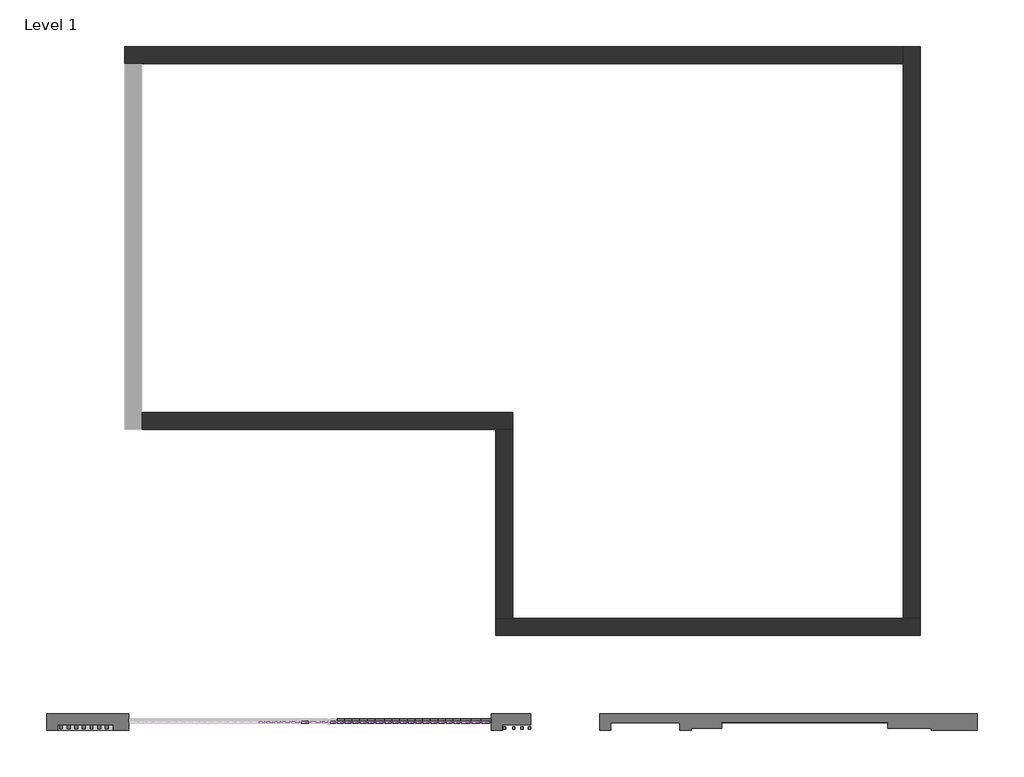
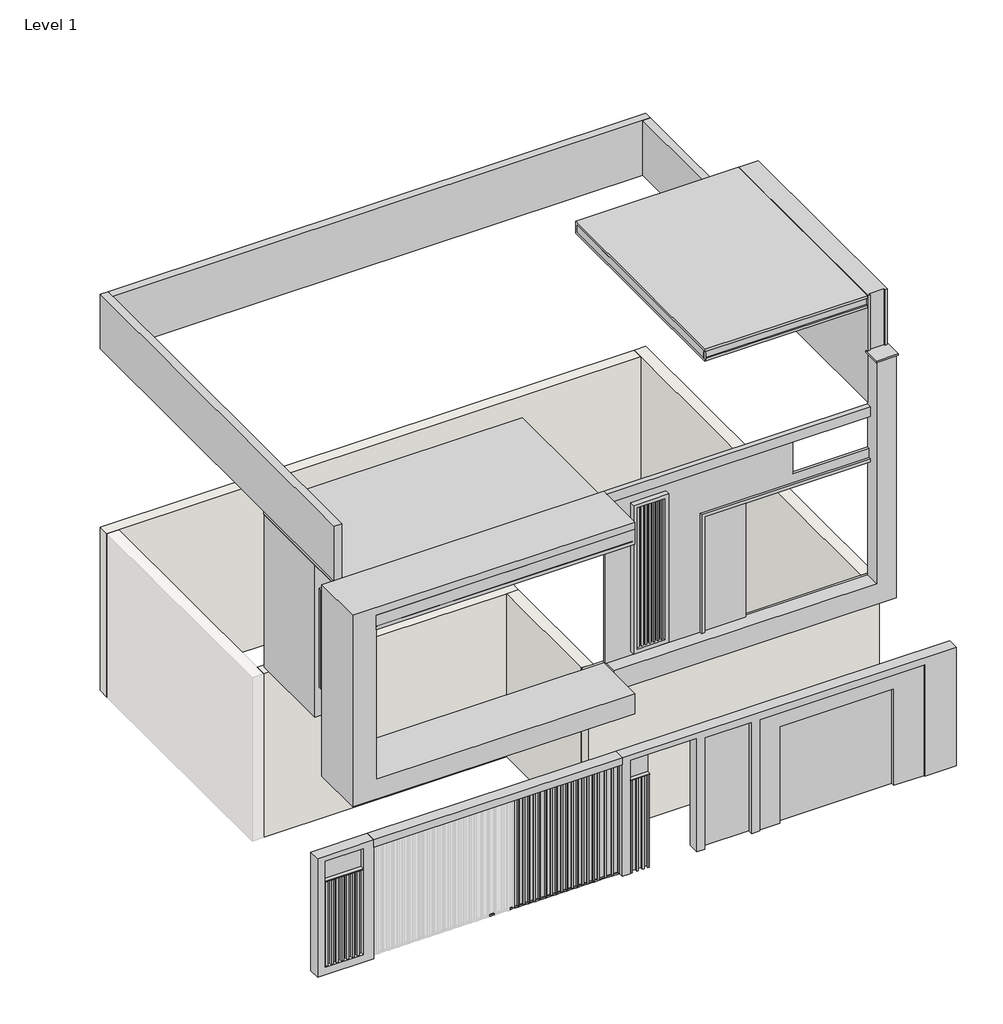
# One storey, part 2 of 2: 68 members, 19 plates, 5 walls, 1 proxy.
"""IFC4 building model written with IfcOpenShell, lengths in millimetres."""

from ifc_helpers import new_model, si_unit, frame, origin, place, context, project, spatial, polyline, outline, extrude, faceted_brep, transform, mapped, element, save
from components import generic_models_1_generic_models_1_ed2606db, member_dc9417da, member_f9b59f6e, member_b36ee676, member_838ad8ec, member_d2c643f7, member_fc53d4cb, member_4ec4fa50, member_7046656e, system_panel_glazed_eef689be, system_panel_glazed_28c5fff6, system_panel_glazed_b538bb1a

model = new_model("IFC4")

# Units and contexts
model_context = context("Model", 3, world=origin())
ifc_project = project(units=[si_unit("LENGTHUNIT", "METRE", prefix="MILLI")], contexts=[model_context])

# Site, building, storey
site = spatial("IfcSite", under=ifc_project)
building = spatial("IfcBuilding", under=site)
storey = spatial("IfcBuildingStorey", under=building, Name="Level 1", Elevation=-304.8)

# Proxy
placement = place(None, origin())
generic_models_1_generic_models_1_shape = generic_models_1_generic_models_1_ed2606db(model_context)
element("IfcBuildingElementProxy", 1, Name="Generic Models 1 : Generic Models 1", ObjectType="Generic Models 1 : Generic Models 1", at=placement, inside=storey, context=model_context, shape_type="MappedRepresentation", body=[
    mapped(generic_models_1_generic_models_1_shape, transform((0.0, 0.0, 0.0), x_axis=(1.0, 0.0, 0.0), y_axis=(0.0, 1.0, 0.0), z_axis=(0.0, 0.0, 1.0))),
])

# Members
member_shape = member_dc9417da(model_context)
element("IfcMember", 2, ObjectType="Rectangular Mullion : 1\" Square", at=placement, inside=storey, context=model_context, shape_type="MappedRepresentation", body=[
    mapped(member_shape, transform((-5007.1379854, -6958.7165974, 1982.7875), x_axis=(0.0, 0.0, 1.0), y_axis=(0.0, -1.0, 0.0), z_axis=(1.0, 0.0, 0.0))),
])
member_2_shape = member_f9b59f6e(model_context)
element("IfcMember", 3, ObjectType="Rectangular Mullion : 1\" Square", at=placement, inside=storey, context=model_context, shape_type="MappedRepresentation", body=[
    mapped(member_2_shape, transform((-6937.5379854, -6958.7165974, -304.8), x_axis=(1.0, 0.0, 0.0), y_axis=(0.0, -1.0, 0.0), z_axis=(0.0, 0.0, -1.0))),
])
element("IfcMember", 4, ObjectType="Rectangular Mullion : 1\" Square", at=placement, inside=storey, context=model_context, shape_type="MappedRepresentation", body=[
    mapped(member_2_shape, transform((-6835.9379854, -6958.7165974, -304.8), x_axis=(1.0, 0.0, 0.0), y_axis=(0.0, -1.0, 0.0), z_axis=(0.0, 0.0, -1.0))),
])
element("IfcMember", 5, ObjectType="Rectangular Mullion : 1\" Square", at=placement, inside=storey, context=model_context, shape_type="MappedRepresentation", body=[
    mapped(member_2_shape, transform((-6734.3379854, -6958.7165974, -304.8), x_axis=(1.0, 0.0, 0.0), y_axis=(0.0, -1.0, 0.0), z_axis=(0.0, 0.0, -1.0))),
])
element("IfcMember", 6, ObjectType="Rectangular Mullion : 1\" Square", at=placement, inside=storey, context=model_context, shape_type="MappedRepresentation", body=[
    mapped(member_2_shape, transform((-6632.7379854, -6958.7165974, -304.8), x_axis=(1.0, 0.0, 0.0), y_axis=(0.0, -1.0, 0.0), z_axis=(0.0, 0.0, -1.0))),
])
element("IfcMember", 7, ObjectType="Rectangular Mullion : 1\" Square", at=placement, inside=storey, context=model_context, shape_type="MappedRepresentation", body=[
    mapped(member_2_shape, transform((-6531.1379854, -6958.7165974, -304.8), x_axis=(1.0, 0.0, 0.0), y_axis=(0.0, -1.0, 0.0), z_axis=(0.0, 0.0, -1.0))),
])
element("IfcMember", 8, ObjectType="Rectangular Mullion : 1\" Square", at=placement, inside=storey, context=model_context, shape_type="MappedRepresentation", body=[
    mapped(member_2_shape, transform((-6404.1379854, -6958.7165974, -304.8), x_axis=(1.0, 0.0, 0.0), y_axis=(0.0, -1.0, 0.0), z_axis=(0.0, 0.0, -1.0))),
])
element("IfcMember", 9, ObjectType="Rectangular Mullion : 1\" Square", at=placement, inside=storey, context=model_context, shape_type="MappedRepresentation", body=[
    mapped(member_2_shape, transform((-6302.5379854, -6958.7165974, -304.8), x_axis=(1.0, 0.0, 0.0), y_axis=(0.0, -1.0, 0.0), z_axis=(0.0, 0.0, -1.0))),
])
element("IfcMember", 10, ObjectType="Rectangular Mullion : 1\" Square", at=placement, inside=storey, context=model_context, shape_type="MappedRepresentation", body=[
    mapped(member_2_shape, transform((-6200.9379854, -6958.7165974, -304.8), x_axis=(1.0, 0.0, 0.0), y_axis=(0.0, -1.0, 0.0), z_axis=(0.0, 0.0, -1.0))),
])
element("IfcMember", 11, ObjectType="Rectangular Mullion : 1\" Square", at=placement, inside=storey, context=model_context, shape_type="MappedRepresentation", body=[
    mapped(member_2_shape, transform((-6099.3379854, -6958.7165974, -304.8), x_axis=(1.0, 0.0, 0.0), y_axis=(0.0, -1.0, 0.0), z_axis=(0.0, 0.0, -1.0))),
])
element("IfcMember", 12, ObjectType="Rectangular Mullion : 1\" Square", at=placement, inside=storey, context=model_context, shape_type="MappedRepresentation", body=[
    mapped(member_2_shape, transform((-5997.7379854, -6958.7165974, -304.8), x_axis=(1.0, 0.0, 0.0), y_axis=(0.0, -1.0, 0.0), z_axis=(0.0, 0.0, -1.0))),
])
element("IfcMember", 13, ObjectType="Rectangular Mullion : 1\" Square", at=placement, inside=storey, context=model_context, shape_type="MappedRepresentation", body=[
    mapped(member_2_shape, transform((-5896.1379854, -6958.7165974, -304.8), x_axis=(1.0, 0.0, 0.0), y_axis=(0.0, -1.0, 0.0), z_axis=(0.0, 0.0, -1.0))),
])
element("IfcMember", 14, ObjectType="Rectangular Mullion : 1\" Square", at=placement, inside=storey, context=model_context, shape_type="MappedRepresentation", body=[
    mapped(member_2_shape, transform((-5794.5379854, -6958.7165974, -304.8), x_axis=(1.0, 0.0, 0.0), y_axis=(0.0, -1.0, 0.0), z_axis=(0.0, 0.0, -1.0))),
])
element("IfcMember", 15, ObjectType="Rectangular Mullion : 1\" Square", at=placement, inside=storey, context=model_context, shape_type="MappedRepresentation", body=[
    mapped(member_2_shape, transform((-5692.9379854, -6958.7165974, -304.8), x_axis=(1.0, 0.0, 0.0), y_axis=(0.0, -1.0, 0.0), z_axis=(0.0, 0.0, -1.0))),
])
element("IfcMember", 16, ObjectType="Rectangular Mullion : 1\" Square", at=placement, inside=storey, context=model_context, shape_type="MappedRepresentation", body=[
    mapped(member_2_shape, transform((-5591.3379854, -6958.7165974, -304.8), x_axis=(1.0, 0.0, 0.0), y_axis=(0.0, -1.0, 0.0), z_axis=(0.0, 0.0, -1.0))),
])
element("IfcMember", 17, ObjectType="Rectangular Mullion : 1\" Square", at=placement, inside=storey, context=model_context, shape_type="MappedRepresentation", body=[
    mapped(member_2_shape, transform((-5489.7379854, -6958.7165974, -304.8), x_axis=(1.0, 0.0, 0.0), y_axis=(0.0, -1.0, 0.0), z_axis=(0.0, 0.0, -1.0))),
])
element("IfcMember", 18, ObjectType="Rectangular Mullion : 1\" Square", at=placement, inside=storey, context=model_context, shape_type="MappedRepresentation", body=[
    mapped(member_2_shape, transform((-5388.1379854, -6958.7165974, -304.8), x_axis=(1.0, 0.0, 0.0), y_axis=(0.0, -1.0, 0.0), z_axis=(0.0, 0.0, -1.0))),
])
element("IfcMember", 19, ObjectType="Rectangular Mullion : 1\" Square", at=placement, inside=storey, context=model_context, shape_type="MappedRepresentation", body=[
    mapped(member_2_shape, transform((-5252.6713187, -6958.7165974, -304.8), x_axis=(1.0, 0.0, 0.0), y_axis=(0.0, -1.0, 0.0), z_axis=(0.0, 0.0, -1.0))),
])
element("IfcMember", 20, ObjectType="Rectangular Mullion : 1\" Square", at=placement, inside=storey, context=model_context, shape_type="MappedRepresentation", body=[
    mapped(member_2_shape, transform((-5117.204652, -6958.7165974, -304.8), x_axis=(1.0, 0.0, 0.0), y_axis=(0.0, -1.0, 0.0), z_axis=(0.0, 0.0, -1.0))),
])
member_3_shape = member_b36ee676(model_context)
element("IfcMember", 21, ObjectType="Rectangular Mullion : 1\" Square", at=placement, inside=storey, context=model_context, shape_type="MappedRepresentation", body=[
    mapped(member_3_shape, transform((-7121.6879854, -6958.7165974, -304.8), x_axis=(0.0, 0.0, -1.0), y_axis=(0.0, -1.0, 0.0), z_axis=(-1.0, 0.0, 0.0))),
])
member_4_shape = member_838ad8ec(model_context)
element("IfcMember", 22, ObjectType="Rectangular Mullion : 1\" Square", at=placement, inside=storey, context=model_context, shape_type="MappedRepresentation", body=[
    mapped(member_4_shape, transform((-7026.4379854, -6958.7165974, -304.8), x_axis=(0.0, 0.0, -1.0), y_axis=(0.0, -1.0, 0.0), z_axis=(-1.0, 0.0, 0.0))),
])
element("IfcMember", 23, ObjectType="Rectangular Mullion : 1\" Square", at=placement, inside=storey, context=model_context, shape_type="MappedRepresentation", body=[
    mapped(member_4_shape, transform((-6924.8379854, -6958.7165974, -304.8), x_axis=(0.0, 0.0, -1.0), y_axis=(0.0, -1.0, 0.0), z_axis=(-1.0, 0.0, 0.0))),
])
element("IfcMember", 24, ObjectType="Rectangular Mullion : 1\" Square", at=placement, inside=storey, context=model_context, shape_type="MappedRepresentation", body=[
    mapped(member_4_shape, transform((-6823.2379854, -6958.7165974, -304.8), x_axis=(0.0, 0.0, -1.0), y_axis=(0.0, -1.0, 0.0), z_axis=(-1.0, 0.0, 0.0))),
])
element("IfcMember", 25, ObjectType="Rectangular Mullion : 1\" Square", at=placement, inside=storey, context=model_context, shape_type="MappedRepresentation", body=[
    mapped(member_4_shape, transform((-6721.6379854, -6958.7165974, -304.8), x_axis=(0.0, 0.0, -1.0), y_axis=(0.0, -1.0, 0.0), z_axis=(-1.0, 0.0, 0.0))),
])
element("IfcMember", 26, ObjectType="Rectangular Mullion : 1\" Square", at=placement, inside=storey, context=model_context, shape_type="MappedRepresentation", body=[
    mapped(member_4_shape, transform((-6620.0379854, -6958.7165974, -304.8), x_axis=(0.0, 0.0, -1.0), y_axis=(0.0, -1.0, 0.0), z_axis=(-1.0, 0.0, 0.0))),
])
element("IfcMember", 27, ObjectType="Rectangular Mullion : 1\" Square", at=placement, inside=storey, context=model_context, shape_type="MappedRepresentation", body=[
    mapped(member_4_shape, transform((-6391.4379854, -6958.7165974, -304.8), x_axis=(0.0, 0.0, -1.0), y_axis=(0.0, -1.0, 0.0), z_axis=(-1.0, 0.0, 0.0))),
])
element("IfcMember", 28, ObjectType="Rectangular Mullion : 1\" Square", at=placement, inside=storey, context=model_context, shape_type="MappedRepresentation", body=[
    mapped(member_4_shape, transform((-6289.8379854, -6958.7165974, -304.8), x_axis=(0.0, 0.0, -1.0), y_axis=(0.0, -1.0, 0.0), z_axis=(-1.0, 0.0, 0.0))),
])
element("IfcMember", 29, ObjectType="Rectangular Mullion : 1\" Square", at=placement, inside=storey, context=model_context, shape_type="MappedRepresentation", body=[
    mapped(member_4_shape, transform((-6188.2379854, -6958.7165974, -304.8), x_axis=(0.0, 0.0, -1.0), y_axis=(0.0, -1.0, 0.0), z_axis=(-1.0, 0.0, 0.0))),
])
element("IfcMember", 30, ObjectType="Rectangular Mullion : 1\" Square", at=placement, inside=storey, context=model_context, shape_type="MappedRepresentation", body=[
    mapped(member_4_shape, transform((-6086.6379854, -6958.7165974, -304.8), x_axis=(0.0, 0.0, -1.0), y_axis=(0.0, -1.0, 0.0), z_axis=(-1.0, 0.0, 0.0))),
])
element("IfcMember", 31, ObjectType="Rectangular Mullion : 1\" Square", at=placement, inside=storey, context=model_context, shape_type="MappedRepresentation", body=[
    mapped(member_4_shape, transform((-5985.0379854, -6958.7165974, -304.8), x_axis=(0.0, 0.0, -1.0), y_axis=(0.0, -1.0, 0.0), z_axis=(-1.0, 0.0, 0.0))),
])
element("IfcMember", 32, ObjectType="Rectangular Mullion : 1\" Square", at=placement, inside=storey, context=model_context, shape_type="MappedRepresentation", body=[
    mapped(member_4_shape, transform((-5883.4379854, -6958.7165974, -304.8), x_axis=(0.0, 0.0, -1.0), y_axis=(0.0, -1.0, 0.0), z_axis=(-1.0, 0.0, 0.0))),
])
element("IfcMember", 33, ObjectType="Rectangular Mullion : 1\" Square", at=placement, inside=storey, context=model_context, shape_type="MappedRepresentation", body=[
    mapped(member_4_shape, transform((-5781.8379854, -6958.7165974, -304.8), x_axis=(0.0, 0.0, -1.0), y_axis=(0.0, -1.0, 0.0), z_axis=(-1.0, 0.0, 0.0))),
])
element("IfcMember", 34, ObjectType="Rectangular Mullion : 1\" Square", at=placement, inside=storey, context=model_context, shape_type="MappedRepresentation", body=[
    mapped(member_4_shape, transform((-5680.2379854, -6958.7165974, -304.8), x_axis=(0.0, 0.0, -1.0), y_axis=(0.0, -1.0, 0.0), z_axis=(-1.0, 0.0, 0.0))),
])
element("IfcMember", 35, ObjectType="Rectangular Mullion : 1\" Square", at=placement, inside=storey, context=model_context, shape_type="MappedRepresentation", body=[
    mapped(member_4_shape, transform((-5578.6379854, -6958.7165974, -304.8), x_axis=(0.0, 0.0, -1.0), y_axis=(0.0, -1.0, 0.0), z_axis=(-1.0, 0.0, 0.0))),
])
element("IfcMember", 36, ObjectType="Rectangular Mullion : 1\" Square", at=placement, inside=storey, context=model_context, shape_type="MappedRepresentation", body=[
    mapped(member_4_shape, transform((-5477.0379854, -6958.7165974, -304.8), x_axis=(0.0, 0.0, -1.0), y_axis=(0.0, -1.0, 0.0), z_axis=(-1.0, 0.0, 0.0))),
])
member_5_shape = member_d2c643f7(model_context)
element("IfcMember", 37, ObjectType="Rectangular Mullion : 1\" Square", at=placement, inside=storey, context=model_context, shape_type="MappedRepresentation", body=[
    mapped(member_5_shape, transform((-7509.0379854, -6958.7165974, -304.8), x_axis=(0.0, 0.0, -1.0), y_axis=(0.0, -1.0, 0.0), z_axis=(-1.0, 0.0, 0.0))),
])
element("IfcMember", 38, ObjectType="Rectangular Mullion : 1\" Square", at=placement, inside=storey, context=model_context, shape_type="MappedRepresentation", body=[
    mapped(member_5_shape, transform((-6518.4379854, -6958.7165974, -304.8), x_axis=(0.0, 0.0, -1.0), y_axis=(0.0, -1.0, 0.0), z_axis=(-1.0, 0.0, 0.0))),
])
member_6_shape = member_fc53d4cb(model_context)
element("IfcMember", 39, ObjectType="Rectangular Mullion : 1\" Square", at=placement, inside=storey, context=model_context, shape_type="MappedRepresentation", body=[
    mapped(member_6_shape, transform((-5375.4379854, -6958.7165974, -304.8), x_axis=(0.0, 0.0, -1.0), y_axis=(0.0, -1.0, 0.0), z_axis=(-1.0, 0.0, 0.0))),
])
element("IfcMember", 40, ObjectType="Rectangular Mullion : 1\" Square", at=placement, inside=storey, context=model_context, shape_type="MappedRepresentation", body=[
    mapped(member_6_shape, transform((-5239.9713187, -6958.7165974, -304.8), x_axis=(0.0, 0.0, -1.0), y_axis=(0.0, -1.0, 0.0), z_axis=(-1.0, 0.0, 0.0))),
])
element("IfcMember", 41, ObjectType="Rectangular Mullion : 1\" Square", at=placement, inside=storey, context=model_context, shape_type="MappedRepresentation", body=[
    mapped(member_shape, transform((-5104.504652, -6958.7165974, -304.8), x_axis=(0.0, 0.0, -1.0), y_axis=(0.0, -1.0, 0.0), z_axis=(-1.0, 0.0, 0.0))),
])
element("IfcMember", 42, ObjectType="Rectangular Mullion : 1\" Square", at=placement, inside=storey, context=model_context, shape_type="MappedRepresentation", body=[
    mapped(member_5_shape, transform((-7407.4379854, -6958.7165974, 1982.7875), x_axis=(0.0, 0.0, 1.0), y_axis=(0.0, -1.0, 0.0), z_axis=(1.0, 0.0, 0.0))),
])
element("IfcMember", 43, ObjectType="Rectangular Mullion : 1\" Square", at=placement, inside=storey, context=model_context, shape_type="MappedRepresentation", body=[
    mapped(member_5_shape, transform((-7661.4379854, -6958.7165974, 1982.7875), x_axis=(0.0, 0.0, 1.0), y_axis=(0.0, -1.0, 0.0), z_axis=(1.0, 0.0, 0.0))),
])
element("IfcMember", 44, ObjectType="Rectangular Mullion : 1\" Square", at=placement, inside=storey, context=model_context, shape_type="MappedRepresentation", body=[
    mapped(member_5_shape, transform((-7534.4379854, -6958.7165974, 1982.7875), x_axis=(0.0, 0.0, 1.0), y_axis=(0.0, -1.0, 0.0), z_axis=(1.0, 0.0, 0.0))),
])
element("IfcMember", 45, ObjectType="Rectangular Mullion : 1\" Square", at=placement, inside=storey, context=model_context, shape_type="MappedRepresentation", body=[
    mapped(member_5_shape, transform((-6416.8379854, -6958.7165974, 1982.7875), x_axis=(0.0, 0.0, 1.0), y_axis=(0.0, -1.0, 0.0), z_axis=(1.0, 0.0, 0.0))),
])
member_7_shape = member_4ec4fa50(model_context)
element("IfcMember", 46, ObjectType="Rectangular Mullion : 1\" Square", at=placement, inside=storey, context=model_context, shape_type="MappedRepresentation", body=[
    mapped(member_7_shape, transform((-7255.0379854, -6958.7165974, 1982.7875), x_axis=(0.0, 0.0, 1.0), y_axis=(0.0, -1.0, 0.0), z_axis=(1.0, 0.0, 0.0))),
])
element("IfcMember", 47, ObjectType="Rectangular Mullion : 1\" Square", at=placement, inside=storey, context=model_context, shape_type="MappedRepresentation", body=[
    mapped(member_4_shape, transform((-7991.6379854, -6958.7165974, 1982.7875), x_axis=(0.0, 0.0, 1.0), y_axis=(0.0, -1.0, 0.0), z_axis=(1.0, 0.0, 0.0))),
])
element("IfcMember", 48, ObjectType="Rectangular Mullion : 1\" Square", at=placement, inside=storey, context=model_context, shape_type="MappedRepresentation", body=[
    mapped(member_4_shape, transform((-7890.0379854, -6958.7165974, 1982.7875), x_axis=(0.0, 0.0, 1.0), y_axis=(0.0, -1.0, 0.0), z_axis=(1.0, 0.0, 0.0))),
])
element("IfcMember", 49, ObjectType="Rectangular Mullion : 1\" Square", at=placement, inside=storey, context=model_context, shape_type="MappedRepresentation", body=[
    mapped(member_4_shape, transform((-7788.4379854, -6958.7165974, 1982.7875), x_axis=(0.0, 0.0, 1.0), y_axis=(0.0, -1.0, 0.0), z_axis=(1.0, 0.0, 0.0))),
])
element("IfcMember", 50, ObjectType="Rectangular Mullion : 1\" Square", at=placement, inside=storey, context=model_context, shape_type="MappedRepresentation", body=[
    mapped(member_4_shape, transform((-6950.2379854, -6958.7165974, 1982.7875), x_axis=(0.0, 0.0, 1.0), y_axis=(0.0, -1.0, 0.0), z_axis=(1.0, 0.0, 0.0))),
])
element("IfcMember", 51, ObjectType="Rectangular Mullion : 1\" Square", at=placement, inside=storey, context=model_context, shape_type="MappedRepresentation", body=[
    mapped(member_4_shape, transform((-6848.6379854, -6958.7165974, 1982.7875), x_axis=(0.0, 0.0, 1.0), y_axis=(0.0, -1.0, 0.0), z_axis=(1.0, 0.0, 0.0))),
])
element("IfcMember", 52, ObjectType="Rectangular Mullion : 1\" Square", at=placement, inside=storey, context=model_context, shape_type="MappedRepresentation", body=[
    mapped(member_4_shape, transform((-6747.0379854, -6958.7165974, 1982.7875), x_axis=(0.0, 0.0, 1.0), y_axis=(0.0, -1.0, 0.0), z_axis=(1.0, 0.0, 0.0))),
])
element("IfcMember", 53, ObjectType="Rectangular Mullion : 1\" Square", at=placement, inside=storey, context=model_context, shape_type="MappedRepresentation", body=[
    mapped(member_4_shape, transform((-6645.4379854, -6958.7165974, 1982.7875), x_axis=(0.0, 0.0, 1.0), y_axis=(0.0, -1.0, 0.0), z_axis=(1.0, 0.0, 0.0))),
])
element("IfcMember", 54, ObjectType="Rectangular Mullion : 1\" Square", at=placement, inside=storey, context=model_context, shape_type="MappedRepresentation", body=[
    mapped(member_4_shape, transform((-6543.8379854, -6958.7165974, 1982.7875), x_axis=(0.0, 0.0, 1.0), y_axis=(0.0, -1.0, 0.0), z_axis=(1.0, 0.0, 0.0))),
])
element("IfcMember", 55, ObjectType="Rectangular Mullion : 1\" Square", at=placement, inside=storey, context=model_context, shape_type="MappedRepresentation", body=[
    mapped(member_4_shape, transform((-6315.2379854, -6958.7165974, 1982.7875), x_axis=(0.0, 0.0, 1.0), y_axis=(0.0, -1.0, 0.0), z_axis=(1.0, 0.0, 0.0))),
])
element("IfcMember", 56, ObjectType="Rectangular Mullion : 1\" Square", at=placement, inside=storey, context=model_context, shape_type="MappedRepresentation", body=[
    mapped(member_4_shape, transform((-6213.6379854, -6958.7165974, 1982.7875), x_axis=(0.0, 0.0, 1.0), y_axis=(0.0, -1.0, 0.0), z_axis=(1.0, 0.0, 0.0))),
])
element("IfcMember", 57, ObjectType="Rectangular Mullion : 1\" Square", at=placement, inside=storey, context=model_context, shape_type="MappedRepresentation", body=[
    mapped(member_4_shape, transform((-6112.0379854, -6958.7165974, 1982.7875), x_axis=(0.0, 0.0, 1.0), y_axis=(0.0, -1.0, 0.0), z_axis=(1.0, 0.0, 0.0))),
])
element("IfcMember", 58, ObjectType="Rectangular Mullion : 1\" Square", at=placement, inside=storey, context=model_context, shape_type="MappedRepresentation", body=[
    mapped(member_4_shape, transform((-6010.4379854, -6958.7165974, 1982.7875), x_axis=(0.0, 0.0, 1.0), y_axis=(0.0, -1.0, 0.0), z_axis=(1.0, 0.0, 0.0))),
])
element("IfcMember", 59, ObjectType="Rectangular Mullion : 1\" Square", at=placement, inside=storey, context=model_context, shape_type="MappedRepresentation", body=[
    mapped(member_4_shape, transform((-5908.8379854, -6958.7165974, 1982.7875), x_axis=(0.0, 0.0, 1.0), y_axis=(0.0, -1.0, 0.0), z_axis=(1.0, 0.0, 0.0))),
])
element("IfcMember", 60, ObjectType="Rectangular Mullion : 1\" Square", at=placement, inside=storey, context=model_context, shape_type="MappedRepresentation", body=[
    mapped(member_4_shape, transform((-5807.2379854, -6958.7165974, 1982.7875), x_axis=(0.0, 0.0, 1.0), y_axis=(0.0, -1.0, 0.0), z_axis=(1.0, 0.0, 0.0))),
])
element("IfcMember", 61, ObjectType="Rectangular Mullion : 1\" Square", at=placement, inside=storey, context=model_context, shape_type="MappedRepresentation", body=[
    mapped(member_4_shape, transform((-5705.6379854, -6958.7165974, 1982.7875), x_axis=(0.0, 0.0, 1.0), y_axis=(0.0, -1.0, 0.0), z_axis=(1.0, 0.0, 0.0))),
])
element("IfcMember", 62, ObjectType="Rectangular Mullion : 1\" Square", at=placement, inside=storey, context=model_context, shape_type="MappedRepresentation", body=[
    mapped(member_4_shape, transform((-5604.0379854, -6958.7165974, 1982.7875), x_axis=(0.0, 0.0, 1.0), y_axis=(0.0, -1.0, 0.0), z_axis=(1.0, 0.0, 0.0))),
])
element("IfcMember", 63, ObjectType="Rectangular Mullion : 1\" Square", at=placement, inside=storey, context=model_context, shape_type="MappedRepresentation", body=[
    mapped(member_4_shape, transform((-5502.4379854, -6958.7165974, 1982.7875), x_axis=(0.0, 0.0, 1.0), y_axis=(0.0, -1.0, 0.0), z_axis=(1.0, 0.0, 0.0))),
])
element("IfcMember", 64, ObjectType="Rectangular Mullion : 1\" Square", at=placement, inside=storey, context=model_context, shape_type="MappedRepresentation", body=[
    mapped(member_4_shape, transform((-5400.8379854, -6958.7165974, 1982.7875), x_axis=(0.0, 0.0, 1.0), y_axis=(0.0, -1.0, 0.0), z_axis=(1.0, 0.0, 0.0))),
])
element("IfcMember", 65, ObjectType="Rectangular Mullion : 1\" Square", at=placement, inside=storey, context=model_context, shape_type="MappedRepresentation", body=[
    mapped(member_3_shape, transform((-7159.7879854, -6958.7165974, 1982.7875), x_axis=(0.0, 0.0, 1.0), y_axis=(0.0, -1.0, 0.0), z_axis=(1.0, 0.0, 0.0))),
])
element("IfcMember", 66, ObjectType="Rectangular Mullion : 1\" Square", at=placement, inside=storey, context=model_context, shape_type="MappedRepresentation", body=[
    mapped(member_3_shape, transform((-7051.8379854, -6958.7165974, 1982.7875), x_axis=(0.0, 0.0, 1.0), y_axis=(0.0, -1.0, 0.0), z_axis=(1.0, 0.0, 0.0))),
])
element("IfcMember", 67, ObjectType="Rectangular Mullion : 1\" Square", at=placement, inside=storey, context=model_context, shape_type="MappedRepresentation", body=[
    mapped(member_6_shape, transform((-5265.3713187, -6958.7165974, 1982.7875), x_axis=(0.0, 0.0, 1.0), y_axis=(0.0, -1.0, 0.0), z_axis=(1.0, 0.0, 0.0))),
])
element("IfcMember", 68, ObjectType="Rectangular Mullion : 1\" Square", at=placement, inside=storey, context=model_context, shape_type="MappedRepresentation", body=[
    mapped(member_6_shape, transform((-5129.904652, -6958.7165974, 1982.7875), x_axis=(0.0, 0.0, 1.0), y_axis=(0.0, -1.0, 0.0), z_axis=(1.0, 0.0, 0.0))),
])
member_8_shape = member_7046656e(model_context)
element("IfcMember", 69, ObjectType="Rectangular Mullion : 1\" Square", at=placement, inside=storey, context=model_context, shape_type="MappedRepresentation", body=[
    mapped(member_8_shape, transform((-4981.7379854, -6958.7165974, -304.8), x_axis=(1.0, 0.0, 0.0), y_axis=(0.0, -1.0, 0.0), z_axis=(0.0, 0.0, -1.0))),
])

# Plates
system_panel_glazed_shape = system_panel_glazed_eef689be(model_context)
element("IfcPlate", 70, ObjectType="System Panel : Glazed", at=placement, inside=storey, context=model_context, shape_type="MappedRepresentation", body=[
    mapped(system_panel_glazed_shape, transform((-6467.6379854, -6958.7165974, -304.8), x_axis=(1.0, 0.0, 0.0), y_axis=(0.0, 1.0, 0.0), z_axis=(0.0, 0.0, 1.0))),
])
system_panel_glazed_2_shape = system_panel_glazed_28c5fff6(model_context)
element("IfcPlate", 71, ObjectType="System Panel : Glazed", at=placement, inside=storey, context=model_context, shape_type="MappedRepresentation", body=[
    mapped(system_panel_glazed_2_shape, transform((-6988.3379854, -6958.7165974, -304.8), x_axis=(1.0, 0.0, 0.0), y_axis=(0.0, 1.0, 0.0), z_axis=(0.0, 0.0, 1.0))),
])
element("IfcPlate", 72, ObjectType="System Panel : Glazed", at=placement, inside=storey, context=model_context, shape_type="MappedRepresentation", body=[
    mapped(system_panel_glazed_2_shape, transform((-6886.7379854, -6958.7165974, -304.8), x_axis=(1.0, 0.0, 0.0), y_axis=(0.0, 1.0, 0.0), z_axis=(0.0, 0.0, 1.0))),
])
element("IfcPlate", 73, ObjectType="System Panel : Glazed", at=placement, inside=storey, context=model_context, shape_type="MappedRepresentation", body=[
    mapped(system_panel_glazed_2_shape, transform((-6785.1379854, -6958.7165974, -304.8), x_axis=(1.0, 0.0, 0.0), y_axis=(0.0, 1.0, 0.0), z_axis=(0.0, 0.0, 1.0))),
])
element("IfcPlate", 74, ObjectType="System Panel : Glazed", at=placement, inside=storey, context=model_context, shape_type="MappedRepresentation", body=[
    mapped(system_panel_glazed_2_shape, transform((-6683.5379854, -6958.7165974, -304.8), x_axis=(1.0, 0.0, 0.0), y_axis=(0.0, 1.0, 0.0), z_axis=(0.0, 0.0, 1.0))),
])
element("IfcPlate", 75, ObjectType="System Panel : Glazed", at=placement, inside=storey, context=model_context, shape_type="MappedRepresentation", body=[
    mapped(system_panel_glazed_2_shape, transform((-6581.9379854, -6958.7165974, -304.8), x_axis=(1.0, 0.0, 0.0), y_axis=(0.0, 1.0, 0.0), z_axis=(0.0, 0.0, 1.0))),
])
element("IfcPlate", 76, ObjectType="System Panel : Glazed", at=placement, inside=storey, context=model_context, shape_type="MappedRepresentation", body=[
    mapped(system_panel_glazed_2_shape, transform((-6353.3379854, -6958.7165974, -304.8), x_axis=(1.0, 0.0, 0.0), y_axis=(0.0, 1.0, 0.0), z_axis=(0.0, 0.0, 1.0))),
])
element("IfcPlate", 77, ObjectType="System Panel : Glazed", at=placement, inside=storey, context=model_context, shape_type="MappedRepresentation", body=[
    mapped(system_panel_glazed_2_shape, transform((-6251.7379854, -6958.7165974, -304.8), x_axis=(1.0, 0.0, 0.0), y_axis=(0.0, 1.0, 0.0), z_axis=(0.0, 0.0, 1.0))),
])
element("IfcPlate", 78, ObjectType="System Panel : Glazed", at=placement, inside=storey, context=model_context, shape_type="MappedRepresentation", body=[
    mapped(system_panel_glazed_2_shape, transform((-6150.1379854, -6958.7165974, -304.8), x_axis=(1.0, 0.0, 0.0), y_axis=(0.0, 1.0, 0.0), z_axis=(0.0, 0.0, 1.0))),
])
element("IfcPlate", 79, ObjectType="System Panel : Glazed", at=placement, inside=storey, context=model_context, shape_type="MappedRepresentation", body=[
    mapped(system_panel_glazed_2_shape, transform((-6048.5379854, -6958.7165974, -304.8), x_axis=(1.0, 0.0, 0.0), y_axis=(0.0, 1.0, 0.0), z_axis=(0.0, 0.0, 1.0))),
])
element("IfcPlate", 80, ObjectType="System Panel : Glazed", at=placement, inside=storey, context=model_context, shape_type="MappedRepresentation", body=[
    mapped(system_panel_glazed_2_shape, transform((-5946.9379854, -6958.7165974, -304.8), x_axis=(1.0, 0.0, 0.0), y_axis=(0.0, 1.0, 0.0), z_axis=(0.0, 0.0, 1.0))),
])
element("IfcPlate", 81, ObjectType="System Panel : Glazed", at=placement, inside=storey, context=model_context, shape_type="MappedRepresentation", body=[
    mapped(system_panel_glazed_2_shape, transform((-5845.3379854, -6958.7165974, -304.8), x_axis=(1.0, 0.0, 0.0), y_axis=(0.0, 1.0, 0.0), z_axis=(0.0, 0.0, 1.0))),
])
element("IfcPlate", 82, ObjectType="System Panel : Glazed", at=placement, inside=storey, context=model_context, shape_type="MappedRepresentation", body=[
    mapped(system_panel_glazed_2_shape, transform((-5743.7379854, -6958.7165974, -304.8), x_axis=(1.0, 0.0, 0.0), y_axis=(0.0, 1.0, 0.0), z_axis=(0.0, 0.0, 1.0))),
])
element("IfcPlate", 83, ObjectType="System Panel : Glazed", at=placement, inside=storey, context=model_context, shape_type="MappedRepresentation", body=[
    mapped(system_panel_glazed_2_shape, transform((-5642.1379854, -6958.7165974, -304.8), x_axis=(1.0, 0.0, 0.0), y_axis=(0.0, 1.0, 0.0), z_axis=(0.0, 0.0, 1.0))),
])
element("IfcPlate", 84, ObjectType="System Panel : Glazed", at=placement, inside=storey, context=model_context, shape_type="MappedRepresentation", body=[
    mapped(system_panel_glazed_2_shape, transform((-5540.5379854, -6958.7165974, -304.8), x_axis=(1.0, 0.0, 0.0), y_axis=(0.0, 1.0, 0.0), z_axis=(0.0, 0.0, 1.0))),
])
element("IfcPlate", 85, ObjectType="System Panel : Glazed", at=placement, inside=storey, context=model_context, shape_type="MappedRepresentation", body=[
    mapped(system_panel_glazed_2_shape, transform((-5438.9379854, -6958.7165974, -304.8), x_axis=(1.0, 0.0, 0.0), y_axis=(0.0, 1.0, 0.0), z_axis=(0.0, 0.0, 1.0))),
])
system_panel_glazed_3_shape = system_panel_glazed_b538bb1a(model_context)
element("IfcPlate", 86, ObjectType="System Panel : Glazed", at=placement, inside=storey, context=model_context, shape_type="MappedRepresentation", body=[
    mapped(system_panel_glazed_3_shape, transform((-5320.404652, -6958.7165974, -304.8), x_axis=(1.0, 0.0, 0.0), y_axis=(0.0, 1.0, 0.0), z_axis=(0.0, 0.0, 1.0))),
])
element("IfcPlate", 87, ObjectType="System Panel : Glazed", at=placement, inside=storey, context=model_context, shape_type="MappedRepresentation", body=[
    mapped(system_panel_glazed_3_shape, transform((-5184.9379854, -6958.7165974, -304.8), x_axis=(1.0, 0.0, 0.0), y_axis=(0.0, 1.0, 0.0), z_axis=(0.0, 0.0, 1.0))),
])
element("IfcPlate", 88, ObjectType="System Panel : Glazed", at=placement, inside=storey, context=model_context, shape_type="MappedRepresentation", body=[
    mapped(system_panel_glazed_3_shape, transform((-5049.4713187, -6958.7165974, -304.8), x_axis=(1.0, 0.0, 0.0), y_axis=(0.0, 1.0, 0.0), z_axis=(0.0, 0.0, 1.0))),
])

# Walls
element("IfcWall", 89, ObjectType="9\" wall", at=placement, inside=storey, context=model_context, shape_type="Brep", body=[
    faceted_brep([(-9858.5379854, 1813.5493179, -304.8), (-9629.9379854, 1813.5493179, -304.8), (504.6620146, 1813.5493179, -304.8), (504.6620146, 1813.5493179, 3048.0), (-9629.9379854, 1813.5493179, 3048.0), (-9858.5379854, 1813.5493179, 3048.0), (-9858.5379854, 2042.1493179, -304.8), (-9858.5379854, 2042.1493179, 3048.0), (504.6620146, 2042.1493179, 3048.0), (504.6620146, 2042.1493179, -304.8)], [[[0, 1, 2, 3, 4, 5]], [[6, 7, 8, 9]], [[2, 1, 0, 6, 9]], [[5, 4, 3, 8, 7]], [[0, 5, 7, 6]], [[3, 2, 9, 8]]]),
])
element("IfcWall", 90, ObjectType="9\" wall", at=placement, inside=storey, context=model_context, shape_type="Brep", body=[
    faceted_brep([(733.2620146, -5577.8506821, -304.8), (504.6620146, -5577.8506821, -304.8), (-4689.6379854, -5577.8506821, -304.8), (-4918.2379854, -5577.8506821, -304.8), (-4918.2379854, -5577.8506821, 3048.0), (-4689.6379854, -5577.8506821, 3048.0), (504.6620146, -5577.8506821, 3048.0), (733.2620146, -5577.8506821, 3048.0), (733.2620146, -5806.4506821, -304.8), (733.2620146, -5806.4506821, 3048.0), (-4918.2379854, -5806.4506821, 3048.0), (-4918.2379854, -5806.4506821, -304.8)], [[[0, 1, 2, 3, 4, 5, 6, 7]], [[8, 9, 10, 11]], [[3, 2, 1, 0, 8, 11]], [[7, 6, 5, 4, 10, 9]], [[0, 7, 9, 8]], [[4, 3, 11, 10]]]),
])
element("IfcWall", 91, ObjectType="9\" wall", at=placement, inside=storey, context=model_context, shape_type="Brep", body=[
    faceted_brep([(504.6620146, 2042.1493179, -304.8), (504.6620146, 1813.5493179, -304.8), (504.6620146, -5577.8506821, -304.8), (504.6620146, -5577.8506821, 3048.0), (504.6620146, 1813.5493179, 3048.0), (504.6620146, 2042.1493179, 3048.0), (733.2620146, 2042.1493179, -304.8), (733.2620146, 2042.1493179, 3048.0), (733.2620146, -5577.8506821, 3048.0), (733.2620146, -5577.8506821, -304.8)], [[[0, 1, 2, 3, 4, 5]], [[6, 7, 8, 9]], [[2, 1, 0, 6, 9]], [[5, 4, 3, 8, 7]], [[0, 5, 7, 6]], [[3, 2, 9, 8]]]),
])
element("IfcWall", 92, ObjectType="9\" wall", at=placement, inside=storey, context=model_context, shape_type="Brep", body=[
    faceted_brep([(-9629.9379854, -3063.2506821, -304.8), (-4918.2379854, -3063.2506821, -304.8), (-4689.6379854, -3063.2506821, -304.8), (-4689.6379854, -3063.2506821, 3048.0), (-4918.2379854, -3063.2506821, 3048.0), (-9629.9379854, -3063.2506821, 3048.0), (-9629.9379854, -2834.6506821, -304.8), (-9629.9379854, -2834.6506821, 3048.0), (-4689.6379854, -2834.6506821, 3048.0), (-4689.6379854, -2834.6506821, -304.8)], [[[0, 1, 2, 3, 4, 5]], [[6, 7, 8, 9]], [[2, 1, 0, 6, 9]], [[5, 4, 3, 8, 7]], [[3, 2, 9, 8]], [[0, 5, 7, 6]]]),
])
element("IfcWall", 93, ObjectType="9\" wall", at=placement, inside=storey, context=model_context, shape_type="SweptSolid", body=[
    extrude(outline(polyline([(-4918.2379854, -5577.8506821), (-4918.2379854, -3063.2506821), (-4689.6379854, -3063.2506821), (-4689.6379854, -5577.8506821), (-4918.2379854, -5577.8506821)])), frame((0.0, 0.0, -304.8), z_axis=(0.0, 0.0, 1.0), x_axis=(1.0, 0.0, 0.0)), (0.0, 0.0, 1.0), 3352.8),
])

save(model, "model.ifc")

# Revit data of these elements
# Type "Rectangular Mullion : 1\" Square"
#   built-in parameter 1007304 = 0.0833333 (stored number, unit not read)
#   built-in parameter 1007301 = 0.0416667 (stored number, unit not read)
#   built-in parameter 1007300 = 0.0416667 (stored number, unit not read)
# Type "System Panel : Glazed"
#   Construction Type Id = "GSP4R"
#   Analytic Construction = "1/8 in Pilkington single glazing"
#   Visual Light Transmittance = 0.9
#   Solar Heat Gain Coefficient = 0.86
#   Heat Transfer Coefficient (U) = 1.18115 BTU/(h·ft²·°F)
#   Define Thermal Properties by = 1
# Type "9\" wall"
#   Assembly Code = "B2010"
# Element 1 (IfcBuildingElementProxy, "Generic Models 1 : Generic Models 1")
#   Phase Created = New Construction
#   Materials on its faces: "door", "Wood - Stained", "balcony wall", "mullions", "black"
# Elements 2, 3, 4, 5, 6, 7, 8, 9, 10, 11, 12, 13, 14, 15, 16, 17, 18, 19, 20, 21, 22, 23, 24, 25, 26, 27, 28, 29, 30, 31, 32, 33, 34, 35, 36, 37, 38, 39, 40, 41, 42, 43, 44, 45, 46, 47, 48, 49, 50, 51, 52, 53, 54, 55, 56, 57, 58, 59, 60, 61, 62, 63, 64, 65, 66, 67, 68, 69 (IfcMember, "Rectangular Mullion : 1\" Square")
#   Phase Created = New Construction
#   Materials on its faces: "black"
# Elements 70, 71, 72, 73, 74, 75, 76, 77, 78, 79, 80, 81, 82, 83, 84, 85, 86, 87, 88 (IfcPlate, "System Panel : Glazed")
#   Phase Created = New Construction
#   Materials on its faces: "Glass"
# Elements 89, 90, 91, 92, 93 (IfcWall, "9\" wall")
#   Top Offset = 0' - 0"
#   Base Offset = 0' - 0"
#   wall height = 11' - 0"
#   Phase Created = New Construction
#   Base Constraint = Level 1
#   Top Constraint = Level 2
# Materials
#   "door": class "Generic", colour RGB 120 120 120, transparency 0, Cost = 0
#   "Wood - Stained": class "Wood", colour RGB 224 178 126, transparency 0, Cost = 0
#   "balcony wall": class "Generic", colour RGB 120 120 120, transparency 0, Cost = 0
#   "mullions": class "Generic", colour RGB 120 120 120, transparency 0, Cost = 0
#   "black": class "Generic", colour RGB 120 120 120, transparency 0, Cost = 0
#   "Glass": class "Glass", colour RGB 0 128 192, transparency 0.75, Description = "Soda Lime Glass", Cost = 0
